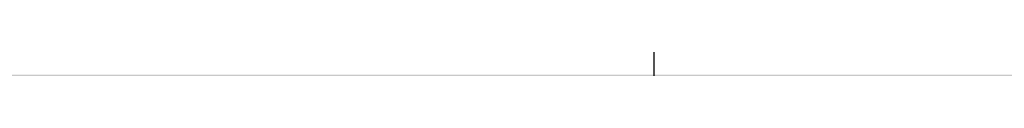
# Model space of a CAD drawing. Units: inches. Extents: x 2083 to 3317, y 1141 to 2115.
# Tile 62 of 256: x 2237.106 to 2238.294, y 1477.769 to 1477.78. Entities that reach past the tile are written whole.
import ezdxf

# ---------------------------------------------------------------- set-up
doc = ezdxf.new("R2010")
doc.units = ezdxf.units.IN
doc.layers.add('A-ANNO-DIMS', color=2, linetype='Continuous', lineweight=18)
doc.layers.add('A-WALL-PATT', color=251, linetype='Continuous', lineweight=13, true_color=0x636466)
doc.styles.get("Standard").update_dxf_attribs({"font": 'arial.ttf'})
doc.dimstyles.new('ISO-25', dxfattribs={"dimtxt": 12, "dimasz": 12, "dimexe": 1.25, "dimexo": 0.625, "dimtad": 1, "dimlunit": 3, "dimtxsty": 'Standard', "dimcen": 2.5, "dimadec": 0, "dimazin": 0, "dimtfac": 1, "dimtmove": 0, "dimatfit": 3, "dimfxl": 1, "dimarcsym": 0})

# ---------------------------------------------------------------- blocks, each defined once
blk = doc.blocks.new('*D30')
at = {"layer": 'A-ANNO-DIMS', "color": 0, "lineweight": -2, "transparency": 16777216}
for p, q in [((2240.0179, 1445.2738), (2240.0179, 1448.0455)), ((2254.3293, 1445.2738), (2254.3293, 1448.0455)), ((2228.0179, 1446.7955), (2216.0179, 1446.7955)), ((2240.0179, 1446.7955), (2254.3293, 1446.7955)), ((2266.3293, 1446.7955), (2413.7649, 1446.7955))]:
    blk.add_line(p, q, dxfattribs=at)
at = {"layer": 'A-ANNO-DIMS', "color": 0, "transparency": 16777216}
for points in [[(2228.0179, 1448.7955), (2228.0179, 1444.7955), (2240.0179, 1446.7955)], [(2266.3293, 1448.7955), (2266.3293, 1444.7955), (2254.3293, 1446.7955)]]:
    blk.add_solid(points, dxfattribs=at)
at = {"layer": 'Defpoints', "color": 0, "transparency": 16777216}
for p in [(2254.3293, 1446.7955), (2240.0179, 1444.6488), (2254.3293, 1444.6488)]:
    blk.add_point(p, dxfattribs=at)
at = {"layer": 'A-ANNO-DIMS', "color": 0, "transparency": 16777216, "insert": (2346.0471, 1453.6252), "char_height": 12, "attachment_point": 5}
blk.add_mtext('WC 1\'-2 1/2" TYP.', dxfattribs=at)
blk = doc.blocks.new('*D31')
at = {"layer": 'A-ANNO-DIMS', "color": 0, "lineweight": -2, "transparency": 16777216}
for p, q in [((2237.8711, 1456.6488), (2237.8711, 1541.9152)), ((2239.3929, 1444.6488), (2236.6211, 1444.6488)), ((2237.8711, 1431.5475), (2237.8711, 1444.6488)), ((2239.3929, 1431.5475), (2236.6211, 1431.5475)), ((2237.8711, 1419.5475), (2237.8711, 1407.5475))]:
    blk.add_line(p, q, dxfattribs=at)
at = {"layer": 'A-ANNO-DIMS', "color": 0, "transparency": 16777216}
for points in [[(2235.8711, 1456.6488), (2239.8711, 1456.6488), (2237.8711, 1444.6488)], [(2235.8711, 1419.5475), (2239.8711, 1419.5475), (2237.8711, 1431.5475)]]:
    blk.add_solid(points, dxfattribs=at)
at = {"layer": 'Defpoints', "color": 0, "transparency": 16777216}
for p in [(2237.8711, 1444.6488), (2240.0179, 1444.6488), (2240.0179, 1431.5475)]:
    blk.add_point(p, dxfattribs=at)
at = {"layer": 'A-ANNO-DIMS', "color": 0, "transparency": 16777216, "insert": (2231.2175, 1505.282), "char_height": 12, "attachment_point": 5, "rotation": 90}
blk.add_mtext('1\'-1" TYP.', dxfattribs=at)
blk = doc.blocks.new('*D45')
at = {"layer": 'A-ANNO-DIMS', "color": 0, "lineweight": -2, "transparency": 16777216}
for p, q in [((2235.9598, 1478.3864), (2235.9598, 1531.3614)), ((2418.9598, 1478.3864), (2418.9598, 1531.3614)), ((2247.9598, 1530.1114), (2406.9598, 1530.1114))]:
    blk.add_line(p, q, dxfattribs=at)
at = {"layer": 'A-ANNO-DIMS', "color": 0, "transparency": 16777216}
for points in [[(2247.9598, 1532.1114), (2247.9598, 1528.1114), (2235.9598, 1530.1114)], [(2406.9598, 1532.1114), (2406.9598, 1528.1114), (2418.9598, 1530.1114)]]:
    blk.add_solid(points, dxfattribs=at)
at = {"layer": 'Defpoints', "color": 0, "transparency": 16777216}
for p in [(2418.9598, 1530.1114), (2235.9598, 1477.7614), (2418.9598, 1477.7614)]:
    blk.add_point(p, dxfattribs=at)
at = {"layer": 'A-ANNO-DIMS', "color": 0, "transparency": 16777216, "insert": (2327.4598, 1536.8673), "char_height": 12, "attachment_point": 5}
blk.add_mtext('15\'-3"', dxfattribs=at)
blk = doc.blocks.new('*D62')
at = {"layer": 'A-ANNO-DIMS', "color": 0, "lineweight": -2, "transparency": 16777216}
for p, q in [((2235.9598, 1469.3864), (2235.9598, 1522.3614)), ((2379.9598, 1469.3864), (2379.9598, 1522.3614)), ((2247.9598, 1521.1114), (2367.9598, 1521.1114))]:
    blk.add_line(p, q, dxfattribs=at)
at = {"layer": 'A-ANNO-DIMS', "color": 0, "transparency": 16777216}
for points in [[(2247.9598, 1523.1114), (2247.9598, 1519.1114), (2235.9598, 1521.1114)], [(2367.9598, 1523.1114), (2367.9598, 1519.1114), (2379.9598, 1521.1114)]]:
    blk.add_solid(points, dxfattribs=at)
at = {"layer": 'Defpoints', "color": 0, "transparency": 16777216}
for p in [(2379.9598, 1521.1114), (2235.9598, 1468.7614), (2379.9598, 1468.7614)]:
    blk.add_point(p, dxfattribs=at)
at = {"layer": 'A-ANNO-DIMS', "color": 0, "transparency": 16777216, "insert": (2307.9598, 1527.8632), "char_height": 12, "attachment_point": 5}
blk.add_mtext('12\'-0"', dxfattribs=at)

msp = doc.modelspace()

# ---------------------------------------------------------------- hatches: boundary and pattern name
at = {"layer": 'A-WALL-PATT'}
h = msp.add_hatch(color=256, dxfattribs=at)
h.dxf.hatch_style = 1
h.paths.add_polyline_path([(3126.9598, 2020.7614), (2748.9598, 2020.7614), (2604.9598, 2020.7614), (2226.9598, 2020.7614), (2226.9598, 1702.7614), (2466.9598, 1702.7614), (2466.9598, 1582.7614), (2418.9598, 1582.7614), (2418.9598, 1477.7614), (2226.9598, 1477.7614), (2226.9598, 1263.2614), (2544.9598, 1263.2614), (2544.9598, 1411.7614), (2604.9598, 1411.7614), (2685.9598, 1411.7614), (2685.9598, 1420.7614), (2604.9598, 1420.7614), (2604.9598, 1573.7614), (2604.9598, 1702.7614), (2604.9598, 2011.7614), (2748.9598, 2011.7614), (2748.9598, 1702.7614), (2862.9598, 1702.7614), (2862.9598, 1621.7614), (2871.9598, 1621.7614), (2871.9598, 1702.7614), (2883.9598, 1702.7614), (2883.9598, 1706.9395, -0.026459), (2883.9598, 1711.7614), (2757.9598, 1711.7614), (2757.9598, 1807.7614), (2787.9598, 1807.7614), (2787.9598, 1812.2614), (2757.9598, 1812.2614), (2757.9598, 2011.7614), (2877.9598, 2011.7614), (2877.9598, 1812.2614), (2847.9598, 1812.2614), (2847.9598, 1807.7614), (2889.8357, 1807.7614), (2889.8357, 1812.2614), (2882.4598, 1812.2614), (2882.4598, 2011.7614), (3117.9598, 2011.7614), (3117.9598, 1812.2614), (2937.8357, 1812.2614), (2937.8357, 1807.7614), (2995.7098, 1807.7614), (2995.7098, 1796.1177), (3000.2098, 1796.1177), (3000.2098, 1807.7614), (3117.9598, 1807.7614), (3117.9598, 1711.7614), (3000.2098, 1711.7614), (3000.2098, 1760.1177), (2998.5727, 1760.1177, -0.020711), (2995.7098, 1760.1177), (2995.7098, 1711.7614), (2931.9598, 1711.7614), (2931.9598, 1702.7614), (3126.9598, 1702.7614)])
h.paths.add_polyline_path([(2471.4598, 2011.7614), (2471.4598, 1810.0114), (2462.7169, 1810.0114), (2462.7169, 1805.5114), (2505.9598, 1805.5114), (2505.9598, 1810.0114), (2475.9598, 1810.0114), (2475.9598, 2011.7614), (2595.9598, 2011.7614), (2595.9598, 1810.0114), (2565.9598, 1810.0114), (2565.9598, 1805.5114), (2595.9598, 1805.5114), (2595.9598, 1711.7614), (2235.9598, 1711.7614), (2235.9598, 1805.5114), (2353.7098, 1805.5114), (2353.7098, 1796.0542), (2358.2098, 1796.0542), (2358.2098, 1805.5114), (2414.7169, 1805.5114), (2414.7169, 1810.0114), (2235.9598, 1810.0114), (2235.9598, 2011.7614)], flags=16)
h.paths.add_polyline_path([(2270.2047, 1994.61), (2270.2047, 1970.61), (2246.2047, 1970.61), (2246.2047, 1994.61)], flags=0)
edge = h.paths.add_edge_path(flags=0)
edge.add_ellipse((2332.0274, 1899.7982), major_axis=(-3.043, 3.043), ratio=0.168252, start_angle=-161.3322, end_angle=-156.3071, ccw=False)
edge.add_ellipse((2333.082, 1898.7435), major_axis=(-1.0546, 1.0546), ratio=0.453532, start_angle=-123.371, end_angle=-94.1591)
edge = h.paths.add_edge_path(flags=0)
edge.add_ellipse((2332.0274, 1968.8763), major_axis=(3.043, 3.043), ratio=0.168252, start_angle=18.6678, end_angle=23.6929)
edge.add_spline(control_points=[(2332.9256, 1970.6911), (2332.2268, 1970.3361), (2330.8937, 1969.6589), (2328.4131, 1970.9321), (2327.2039, 1967.7487), (2324.7096, 1969.9556), (2322.5328, 1967.0124), (2320.0128, 1971.2958), (2317.6803, 1968.1578), (2316.0405, 1967.102), (2315.4269, 1966.8096)], knot_values=[0, 0, 0, 0, 2.267059, 4.324559, 6.685584, 8.878641, 11.121502, 14.300359, 17.755284, 19.732645, 19.732645, 19.732645, 19.732645], degree=3, periodic=0)
edge.add_ellipse((2332.0274, 1968.8763), major_axis=(3.043, 3.043), ratio=0.168252, start_angle=18.6678, end_angle=23.6929, ccw=False)
edge.add_ellipse((2333.082, 1969.9309), major_axis=(1.0546, 1.0546), ratio=0.453532, start_angle=56.629, end_angle=85.8409, ccw=False)
edge = h.paths.add_edge_path(flags=0)
edge.add_spline(control_points=[(2296.4283, 1967.9879), (2293.6278, 1965.3363), (2287.7036, 1959.7271), (2299.7439, 1949.9957), (2294.5326, 1935.6685), (2290.5732, 1920.6035), (2293.3941, 1909.9737), (2296.1854, 1904.9665)], knot_values=[0.099185, 0.099185, 0.099185, 0.099185, 0.345301, 0.619822, 0.982653, 1.386093, 1.810555, 1.810555, 1.810555, 1.810555], degree=3, periodic=0)
edge.add_spline(control_points=[(2296.1854, 1904.9665), (2297.3836, 1902.6193), (2298.001, 1901.9493), (2298.553, 1901.4682)], knot_values=[0.006246, 0.006246, 0.006246, 0.006246, 0.055476, 0.055476, 0.055476, 0.055476], degree=3, periodic=0)
edge.add_spline(control_points=[(2298.553, 1901.4682), (2297.2586, 1900.9232), (2295.2253, 1900.2321), (2293.0602, 1900.6142), (2292.1014, 1900.7884), (2292.0896, 1900.7906)], knot_values=[0.312835, 0.312835, 0.312835, 0.312835, 0.40178, 0.474987, 0.475903, 0.475903, 0.475903, 0.475903], degree=3, periodic=0)
edge.add_arc((2292.7936, 1904.6641), 3.937, 215.4209, 259.6982, ccw=False)
edge.add_spline(control_points=[(2289.5853, 1902.3823), (2289.4767, 1902.5351), (2289.3685, 1902.688), (2289.2609, 1902.8412)], knot_values=[0.102872, 0.102872, 0.102872, 0.102872, 0.116896, 0.116896, 0.116896, 0.116896], degree=3, periodic=0)
edge.add_spline(control_points=[(2289.2609, 1902.8412), (2288.6866, 1902.5502), (2287.64, 1902.0199), (2285.8813, 1901.874), (2283.853, 1901.5044), (2281.72, 1899.7105), (2278.467, 1899.4929), (2276.1571, 1901.8832), (2272.259, 1899.8041), (2267.7776, 1901.8432), (2262.2439, 1900.184), (2257.4149, 1901.7821), (2254.3184, 1900.7261), (2253.1783, 1900.3373)], knot_values=[0, 0, 0, 0, 1.907977, 3.477176, 5.261074, 7.972851, 11.680248, 13.717921, 16.939592, 22.789562, 27.502503, 33.595215, 37.145618, 37.145618, 37.145618, 37.145618], degree=3, periodic=0)
edge.add_line((2253.1783, 1900.3373), (2250.2442, 1902.8412))
edge.add_line((2250.2442, 1902.8412), (2250.2442, 1965.8333))
edge.add_line((2250.2442, 1965.8333), (2253.1783, 1968.3371))
edge.add_spline(control_points=[(2253.1783, 1968.3371), (2254.3184, 1967.9483), (2257.4149, 1966.8924), (2262.2439, 1968.4904), (2267.7776, 1966.8313), (2271.5267, 1968.5372), (2273.8759, 1967.8283), (2274.2067, 1967.7276)], knot_values=[0, 0, 0, 0, 0.09018, 0.244935, 0.364644, 0.513233, 0.537855, 0.537855, 0.537855, 0.537855], degree=3, periodic=0)
edge.add_arc((2274.3529, 1963.7933), 3.937, 72.0511, 92.1279, ccw=False)
edge.add_arc((2281.2969, 1985.23), 18.5963, 252.05113, 288.56572)
edge.add_arc((2292.3167, 1956.0289), 12.6461, 71.02679, 113.77822, ccw=False)
edge = h.paths.add_edge_path(flags=0)
edge.add_spline(control_points=[(2274.8994, 1951.8562), (2275.0662, 1951.6166), (2275.2327, 1951.3766), (2275.398, 1951.1359)], knot_values=[1.409916, 1.409916, 1.409916, 1.409916, 1.43159, 1.43159, 1.43159, 1.43159], degree=3, periodic=0)
edge.add_spline(control_points=[(2275.398, 1951.1359), (2275.7921, 1950.5619), (2276.1792, 1949.9838), (2276.5455, 1949.3971)], knot_values=[1.358238, 1.358238, 1.358238, 1.358238, 1.409916, 1.409916, 1.409916, 1.409916], degree=3, periodic=0)
edge.add_line((2276.5455, 1949.3971), (2277.4373, 1947.8622))
edge.add_spline(control_points=[(2277.4373, 1947.8622), (2276.3038, 1945.6731), (2274.6397, 1942.4269), (2274.6316, 1938.0939), (2272.7991, 1930.8515), (2274.3564, 1943.897), (2275.9477, 1947.9234), (2276.5455, 1949.3971)], knot_values=[0.005632, 0.005632, 0.005632, 0.005632, 0.186014, 0.266002, 0.357087, 0.59639, 0.739732, 0.739732, 0.739732, 0.739732], degree=3, periodic=0)
edge.add_spline(control_points=[(2276.5455, 1949.3971), (2276.1792, 1949.9838), (2275.7921, 1950.5619), (2275.398, 1951.1359)], knot_values=[1.358238, 1.358238, 1.358238, 1.358238, 1.409916, 1.409916, 1.409916, 1.409916], degree=3, periodic=0)
edge.add_spline(control_points=[(2275.398, 1951.1359), (2274.9425, 1950.0805), (2274.2078, 1948.0253), (2273.9346, 1944.8515), (2272.4685, 1937.6275), (2273.4662, 1945.6965), (2274.7006, 1951.0595), (2274.8994, 1951.8562)], knot_values=[0.104364, 0.104364, 0.104364, 0.104364, 0.189636, 0.269624, 0.36071, 0.600013, 0.644622, 0.644622, 0.644622, 0.644622], degree=3, periodic=0)
h.paths.add_polyline_path([(2269.1675, 1963.1276, -0.357527), (2268.1706, 1960.9764, -0.092561), (2268.1706, 1939.4363, -0.357527), (2269.1675, 1937.2851, -0.357527), (2267.0163, 1938.282, -0.164785), (2254.6856, 1938.282, -0.357527), (2252.5344, 1937.2851, -0.357527), (2253.5313, 1939.4363, -0.092561), (2253.5313, 1960.9764, -0.357527), (2252.5344, 1963.1276, -0.357527), (2254.6856, 1962.1307, -0.164785), (2267.0163, 1962.1307, -0.357527)], flags=0)
h.paths.add_polyline_path([(2248.8741, 1967.8018), (2248.8741, 1957.0277), (2249.4578, 1957.0277), (2249.4578, 1911.6468), (2248.8741, 1911.6468), (2248.8741, 1900.8727), (2246.5119, 1900.8727, 0.197327), (2244.1497, 1902.4569), (2244.1497, 1966.2176, 0.197327), (2246.5119, 1967.8018)], flags=0)
h.paths.add_polyline_path([(2269.1675, 1931.3893, -0.357527), (2268.1706, 1929.2381, -0.092561), (2268.1706, 1907.6981, -0.357527), (2269.1675, 1905.5469, -0.357527), (2267.0163, 1906.5438, -0.164785), (2254.6856, 1906.5438, -0.357527), (2252.5344, 1905.5469, -0.357527), (2253.5313, 1907.6981, -0.092561), (2253.5313, 1929.2381, -0.357527), (2252.5344, 1931.3893, -0.357527), (2254.6856, 1930.3925, -0.164785), (2267.0163, 1930.3925, -0.357527)], flags=0)
edge = h.paths.add_edge_path(flags=0)
edge.add_spline(control_points=[(2276.1969, 1906.7237), (2276.1681, 1909.0289), (2276.114, 1913.3719), (2270.5984, 1924.925), (2273.9052, 1919.0128), (2275.9217, 1916.2621), (2275.4746, 1912.4021), (2277.2579, 1910.3806), (2276.696, 1908.225), (2276.6462, 1906.813), (2276.6178, 1906.0084)], knot_values=[0, 0, 0, 0, 8.61026, 16.221274, 18.843057, 23.804898, 27.440828, 29.356102, 31.203478, 33.650687, 33.650687, 33.650687, 33.650687], degree=3, periodic=0)
edge.add_spline(control_points=[(2276.6178, 1906.0084), (2276.6233, 1905.6241), (2276.4977, 1904.6287), (2275.4418, 1903.8547), (2274.9373, 1903.0804), (2274.8591, 1902.8412)], knot_values=[0.156488, 0.156488, 0.156488, 0.156488, 0.184398, 0.231376, 0.250598, 0.250598, 0.250598, 0.250598], degree=3, periodic=0)
edge.add_line((2274.8591, 1902.8412), (2276.506, 1902.8412))
edge.add_spline(control_points=[(2276.506, 1902.8412), (2276.7883, 1903.0849), (2277.6651, 1904.1252), (2278.2495, 1904.3407), (2277.6539, 1908.5274), (2278.1557, 1906.2278), (2278.1005, 1905.2859), (2278.8467, 1904.069), (2277.8568, 1903.4149), (2277.8742, 1902.991), (2277.9036, 1902.8412)], knot_values=[0.059574, 0.059574, 0.059574, 0.059574, 0.080753, 0.103741, 0.16972, 0.176036, 0.207137, 0.240474, 0.262341, 0.27366, 0.27366, 0.27366, 0.27366], degree=3, periodic=0)
edge.add_line((2277.9036, 1902.8412), (2280.0298, 1902.8412))
edge.add_spline(control_points=[(2280.0298, 1902.8412), (2279.8882, 1903.0884), (2279.4993, 1903.9816), (2280.1523, 1905.9393), (2278.1036, 1909.6578), (2279.7624, 1907.1853), (2280.3279, 1904.8749), (2280.4851, 1903.4896), (2281.4633, 1903.2494), (2281.7583, 1902.9365), (2281.834, 1902.8412)], knot_values=[0.013856, 0.013856, 0.013856, 0.013856, 0.034874, 0.088867, 0.107879, 0.126738, 0.158714, 0.193757, 0.217487, 0.226722, 0.226722, 0.226722, 0.226722], degree=3, periodic=0)
edge.add_spline(control_points=[(2281.834, 1902.8412), (2281.7875, 1902.8267), (2281.647, 1902.783), (2281.3955, 1902.8595), (2281.0881, 1902.9852), (2280.7207, 1903.0609), (2280.3335, 1903.0257), (2280.1248, 1902.8989), (2280.0298, 1902.8412)], knot_values=[0, 0, 0, 0, 0.14413, 0.435517, 0.749276, 1.153046, 1.548371, 1.878348, 1.878348, 1.878348, 1.878348], degree=3, periodic=0)
edge.add_line((2280.0298, 1902.8412), (2277.9036, 1902.8412))
edge.add_spline(control_points=[(2277.9036, 1902.8412), (2277.8929, 1902.7959), (2277.8654, 1902.6796), (2277.6075, 1902.6875), (2277.2741, 1902.8007), (2276.8379, 1902.6198), (2276.5838, 1902.7893), (2276.506, 1902.8412)], knot_values=[0, 0, 0, 0, 0.127189, 0.326199, 0.628009, 1.24357, 1.515331, 1.515331, 1.515331, 1.515331], degree=3, periodic=0)
edge.add_line((2276.506, 1902.8412), (2274.8591, 1902.8412))
edge.add_spline(control_points=[(2274.8591, 1902.8412), (2274.8144, 1902.8986), (2274.7251, 1903.0134), (2274.4935, 1903.119), (2274.2443, 1902.9605), (2273.9371, 1903.1849), (2273.614, 1902.9831), (2273.4083, 1902.883), (2273.3223, 1902.8412)], knot_values=[0, 0, 0, 0, 0.21843, 0.436957, 0.687977, 0.990379, 1.398396, 1.69185, 1.69185, 1.69185, 1.69185], degree=3, periodic=0)
edge.add_spline(control_points=[(2273.3223, 1902.8412), (2273.6167, 1903.4457), (2274.274, 1904.5383), (2276.0272, 1904.5737), (2276.207, 1906.5836), (2276.1969, 1906.7237)], knot_values=[0.012227, 0.012227, 0.012227, 0.012227, 0.059472, 0.106218, 0.134458, 0.134458, 0.134458, 0.134458], degree=3, periodic=0)
h.paths.add_polyline_path([(2270.7761, 1897.7898), (2270.7761, 1873.7898), (2246.7761, 1873.7898), (2246.7761, 1897.7898)], flags=0)
h.paths.add_polyline_path([(2353.7098, 1760.0051), (2353.7098, 1760.0542), (2358.2098, 1760.0542, -0.033729)], flags=0)
h.paths.add_polyline_path([(2321.8191, 1737.5292), (2341.9953, 1737.5292, -0.414214), (2343.2033, 1736.3212), (2343.2033, 1721.0206, -0.414214), (2341.9953, 1719.8127), (2321.8191, 1719.8127, -0.414214), (2320.6112, 1721.0206), (2320.6112, 1736.3212, -0.414214)], flags=0)
h.paths.add_polyline_path([(2324.235, 1736.3212), (2339.5794, 1736.3212, -0.414214), (2341.9953, 1733.9053), (2341.9953, 1725.4497, -0.414214), (2339.5794, 1723.0338), (2333.6806, 1723.0338), (2333.8453, 1722.0455, -0.870646), (2335.4254, 1721.8259, -0.767327), (2333.9227, 1721.4232), (2331.291, 1721.4232, -0.767327), (2329.7883, 1721.8259, -0.870646), (2331.3684, 1722.0455), (2331.5331, 1723.0338), (2324.235, 1723.0338, -0.414214), (2321.8191, 1725.4497), (2321.8191, 1733.9053, -0.414214)], flags=0)
h.paths.add_polyline_path([(2570.4838, 1928.6154), (2589.6838, 1928.6154), (2590.1688, 1928.6154), (2590.1688, 1904.9934), (2570.4838, 1904.9934)], flags=0)
h.paths.add_polyline_path([(2574.4473, 1927.2638, -1), (2572.8288, 1927.2638, -1)], flags=0)
h.paths.add_polyline_path([(2573.0899, 1926.9409), (2573.925, 1927.776), (2574.1477, 1927.5533), (2573.3126, 1926.7182)], flags=0)
h.paths.add_polyline_path([(2578.7791, 1919.7296, -1), (2571.5917, 1919.7296, -1)], flags=0)
h.paths.add_polyline_path([(2578.3854, 1919.7296, -1), (2571.9854, 1919.7296, -1)], flags=0)
h.paths.add_polyline_path([(2331.5958, 1729.4762, -1), (2333.618, 1729.4762, -1)], flags=0)
h.paths.add_polyline_path([(2578.0342, 1927.2638, -1), (2576.4157, 1927.2638, -1)], flags=0)
h.paths.add_polyline_path([(2576.6889, 1927.5311), (2576.9116, 1927.7538), (2577.7467, 1926.9186), (2577.524, 1926.6959)], flags=0)
h.paths.add_polyline_path([(2578.1391, 1909.8595, -1), (2572.2317, 1909.8595, -1)], flags=0)
h.paths.add_polyline_path([(2577.7454, 1909.8595, -1), (2572.6254, 1909.8595, -1)], flags=0)
h.paths.add_polyline_path([(2583.7977, 1927.2638, -1), (2582.1792, 1927.2638, -1)], flags=0)
h.paths.add_polyline_path([(2582.7186, 1927.7538), (2583.5538, 1926.9186), (2583.3311, 1926.6959), (2582.4959, 1927.5311)], flags=0)
h.paths.add_polyline_path([(2582.4959, 1927.5311), (2582.7186, 1927.7538), (2583.5538, 1926.9186), (2583.3311, 1926.6959)], flags=0)
h.paths.add_polyline_path([(2587.7391, 1920.5296, -1), (2581.8317, 1920.5296, -1)], flags=0)
h.paths.add_polyline_path([(2587.3454, 1920.5296, -1), (2582.2254, 1920.5296, -1)], flags=0)
h.paths.add_polyline_path([(2587.3846, 1927.2638, -1), (2585.7661, 1927.2638, -1)], flags=0)
h.paths.add_polyline_path([(2586.082, 1926.9802), (2586.9172, 1927.8154), (2587.1399, 1927.5927), (2586.3047, 1926.7575)], flags=0)
h.paths.add_polyline_path([(2588.3791, 1910.6595, -1), (2581.1917, 1910.6595, -1)], flags=0)
h.paths.add_polyline_path([(2587.9854, 1910.6595, -1), (2581.5854, 1910.6595, -1)], flags=0)
h.paths.add_polyline_path([(2417.1677, 1729.4779), (2437.3439, 1729.4779, -0.414214), (2438.5519, 1728.2699), (2438.5519, 1712.9693, -0.414214), (2437.3439, 1711.7614), (2417.1677, 1711.7614, -0.414214), (2415.9598, 1712.9693), (2415.9598, 1728.2699, -0.414214)], flags=0)
h.paths.add_polyline_path([(2419.5836, 1728.2699), (2434.928, 1728.2699, -0.414214), (2437.3439, 1725.8541), (2437.3439, 1717.3984, -0.414214), (2434.928, 1714.9825), (2429.0292, 1714.9825), (2429.1939, 1713.9942, -0.870646), (2430.774, 1713.7746, -0.767327), (2429.2713, 1713.372), (2426.6396, 1713.372, -0.767327), (2425.1369, 1713.7746, -0.870646), (2426.717, 1713.9942), (2426.8817, 1714.9825), (2419.5836, 1714.9825, -0.414214), (2417.1677, 1717.3984), (2417.1677, 1725.8541, -0.414214)], flags=0)
h.paths.add_polyline_path([(2419.5836, 1728.2699), (2434.928, 1728.2699, -0.414214), (2437.3439, 1725.8541), (2437.3439, 1717.3984, -0.414214), (2434.928, 1714.9825), (2429.0292, 1714.9825), (2428.3581, 1719.009), (2427.5528, 1719.009), (2426.8817, 1714.9825), (2419.5836, 1714.9825, -0.414214), (2417.1677, 1717.3984), (2417.1677, 1725.8541, -0.414214)], flags=0)
h.paths.add_polyline_path([(2426.9444, 1721.4249, -1), (2428.9666, 1721.4249, -1)], flags=0)
h.paths.add_polyline_path([(2475.9598, 1702.7614), (2595.9598, 1702.7614), (2595.9598, 1582.7614), (2475.9598, 1582.7614)], flags=16)
h.paths.add_polyline_path([(2427.9598, 1573.7614), (2595.9598, 1573.7614), (2595.9598, 1468.7614), (2595.9598, 1420.7614), (2384.4598, 1420.7614), (2384.4598, 1468.7614), (2427.9598, 1468.7614)], flags=16)
h.paths.add_polyline_path([(2379.9598, 1468.7614), (2379.9598, 1420.7614), (2235.9598, 1420.7614), (2235.9598, 1468.7614)], flags=16)
h.paths.add_polyline_path([(2317.816, 1466.6958), (2337.9922, 1466.6958, -0.414214), (2339.2002, 1465.4878), (2339.2002, 1450.1872, -0.414214), (2337.9922, 1448.9792), (2317.816, 1448.9792, -0.414214), (2316.6081, 1450.1872), (2316.6081, 1465.4878, -0.414214)], flags=0)
h.paths.add_polyline_path([(2320.2319, 1465.4878), (2335.5763, 1465.4878, -0.414214), (2337.9922, 1463.0719), (2337.9922, 1454.6163, -0.414214), (2335.5763, 1452.2004), (2329.6775, 1452.2004), (2329.8422, 1451.212, -0.870646), (2331.4223, 1450.9925, -0.767327), (2329.9196, 1450.5898), (2327.2879, 1450.5898, -0.767327), (2325.7852, 1450.9925, -0.870646), (2327.3653, 1451.212), (2327.53, 1452.2004), (2320.2319, 1452.2004, -0.414214), (2317.816, 1454.6163), (2317.816, 1463.0719, -0.414214)], flags=0)
h.paths.add_polyline_path([(2320.2319, 1465.4878), (2335.5763, 1465.4878, -0.414214), (2337.9922, 1463.0719), (2337.9922, 1454.6163, -0.414214), (2335.5763, 1452.2004), (2329.6775, 1452.2004), (2329.0064, 1456.2269), (2328.2011, 1456.2269), (2327.53, 1452.2004), (2320.2319, 1452.2004, -0.414214), (2317.816, 1454.6163), (2317.816, 1463.0719, -0.414214)], flags=0)
h.paths.add_polyline_path([(2327.5926, 1458.6428, -1), (2329.6148, 1458.6428, -1)], flags=0)
h.paths.add_polyline_path([(2244.4117, 1433.3405), (2241.9209, 1433.3405, -0.414214), (2240.0179, 1435.2435), (2240.0179, 1440.9528, -0.414211), (2241.9209, 1442.8559), (2244.4117, 1442.8559, -1.976472)], flags=0)
h.paths.add_polyline_path([(2245.3569, 1434.3975, -0.414214), (2245.3569, 1441.7988, -2.144098)], flags=0)
h.paths.add_polyline_path([(2535.9598, 1416.2614), (2535.9598, 1272.2614), (2235.9598, 1272.2614), (2235.9598, 1416.2614)], flags=16)
h.paths.add_polyline_path([(2260.1196, 1384.2928), (2260.1196, 1362.0386), (2237.8654, 1362.0386), (2237.8654, 1384.2928)], flags=0)
edge = h.paths.add_edge_path(flags=0)
edge.add_line((2318.2518, 1362.0933), (2318.1458, 1362.001))
edge.add_ellipse((2317.4451, 1360.431), major_axis=(2.8216, 2.8216), ratio=0.168252, start_angle=18.6678, end_angle=20.9481, ccw=False)
edge.add_ellipse((2318.423, 1361.409), major_axis=(0.9779, 0.9779), ratio=0.453532, start_angle=56.629, end_angle=70.2262, ccw=False)
edge = h.paths.add_edge_path(flags=0)
edge.add_line((2319.1074, 1295.5711), (2319.015, 1295.6771))
edge.add_ellipse((2317.4451, 1296.3778), major_axis=(-2.8216, 2.8216), ratio=0.168252, start_angle=-161.3322, end_angle=-159.0519, ccw=False)
edge.add_ellipse((2318.423, 1295.3999), major_axis=(-0.9779, 0.9779), ratio=0.453532, start_angle=-123.371, end_angle=-109.7738)
edge = h.paths.add_edge_path(flags=0)
edge.add_spline(control_points=[(2284.2103, 1301.1702), (2284.5807, 1300.4447), (2284.8912, 1299.892), (2285.1596, 1299.461)], knot_values=[0.039066, 0.039066, 0.039066, 0.039066, 0.055476, 0.055476, 0.055476, 0.055476], degree=3, periodic=0)
edge.add_line((2285.1596, 1299.461), (2284.2103, 1301.1702))
edge = h.paths.add_edge_path(flags=0)
edge.add_line((2280.4125, 1297.298), (2283.37, 1297.0361))
edge.add_line((2283.37, 1297.0361), (2286.4057, 1297.9263))
edge.add_spline(control_points=[(2286.4057, 1297.9263), (2285.3055, 1297.4631), (2284.3448, 1297.1292), (2283.37, 1297.0361)], knot_values=[0.394369, 0.394369, 0.394369, 0.394369, 0.475903, 0.475903, 0.475903, 0.475903], degree=3, periodic=0)
edge.add_spline(control_points=[(2283.37, 1297.0361), (2283.2814, 1297.0277), (2282.3163, 1296.9573), (2281.3125, 1297.1345), (2280.4234, 1297.296), (2280.4125, 1297.298)], knot_values=[0.312835, 0.312835, 0.312835, 0.312835, 0.320246, 0.393453, 0.394369, 0.394369, 0.394369, 0.394369], degree=3, periodic=0)
edge = h.paths.add_edge_path(flags=0)
edge.add_line((2284.4356, 1359.6073), (2280.4463, 1355.328))
edge.add_line((2280.4463, 1355.328), (2279.58, 1351.0178))
edge.add_line((2279.58, 1351.0178), (2282.413, 1346.5804))
edge.add_spline(control_points=[(2282.413, 1346.5804), (2283.1533, 1345.5892), (2284.2529, 1344.0289), (2284.801, 1342.3872), (2284.9352, 1341.8055)], knot_values=[1.240098, 1.240098, 1.240098, 1.240098, 1.332892, 1.382712, 1.382712, 1.382712, 1.382712], degree=3, periodic=0)
edge.add_spline(control_points=[(2284.9352, 1341.8055), (2285.3191, 1340.1406), (2285.233, 1338.4092), (2284.9099, 1336.6541)], knot_values=[1.097484, 1.097484, 1.097484, 1.097484, 1.240098, 1.240098, 1.240098, 1.240098], degree=3, periodic=0)
edge.add_spline(control_points=[(2284.9099, 1336.6541), (2284.5868, 1334.899), (2284.0267, 1333.1203), (2283.4626, 1331.3606)], knot_values=[0.95487, 0.95487, 0.95487, 0.95487, 1.097484, 1.097484, 1.097484, 1.097484], degree=3, periodic=0)
edge.add_line((2283.4626, 1331.3606), (2281.8904, 1326.1534))
edge.add_line((2281.8904, 1326.1534), (2280.7563, 1321.0561))
edge.add_line((2280.7563, 1321.0561), (2280.2992, 1316.002))
edge.add_line((2280.2992, 1316.002), (2280.7159, 1310.9501))
edge.add_line((2280.7159, 1310.9501), (2282.0281, 1305.9721))
edge.add_line((2282.0281, 1305.9721), (2284.2103, 1301.1702))
edge.add_spline(control_points=[(2284.2103, 1301.1702), (2283.3407, 1302.7302), (2282.6119, 1304.3365), (2282.0281, 1305.9721)], knot_values=[0.099185, 0.099185, 0.099185, 0.099185, 0.241799, 0.241799, 0.241799, 0.241799], degree=3, periodic=0)
edge.add_spline(control_points=[(2282.0281, 1305.9721), (2281.4443, 1307.6078), (2281.0055, 1309.2728), (2280.7159, 1310.9501)], knot_values=[0.241799, 0.241799, 0.241799, 0.241799, 0.384413, 0.384413, 0.384413, 0.384413], degree=3, periodic=0)
edge.add_spline(control_points=[(2280.7159, 1310.9501), (2280.4332, 1312.5876), (2280.2894, 1314.277), (2280.2989, 1315.962), (2280.2992, 1316.002)], knot_values=[0.384413, 0.384413, 0.384413, 0.384413, 0.523647, 0.527028, 0.527028, 0.527028, 0.527028], degree=3, periodic=0)
edge.add_spline(control_points=[(2280.2992, 1316.002), (2280.3123, 1317.687), (2280.4779, 1319.3679), (2280.7563, 1321.0561)], knot_values=[0.527028, 0.527028, 0.527028, 0.527028, 0.669642, 0.669642, 0.669642, 0.669642], degree=3, periodic=0)
edge.add_spline(control_points=[(2280.7563, 1321.0561), (2281.0346, 1322.7443), (2281.4259, 1324.4396), (2281.8904, 1326.1534)], knot_values=[0.669642, 0.669642, 0.669642, 0.669642, 0.812256, 0.812256, 0.812256, 0.812256], degree=3, periodic=0)
edge.add_spline(control_points=[(2281.8904, 1326.1534), (2282.2644, 1327.5333), (2282.7879, 1329.2618), (2283.3528, 1331.0178), (2283.4626, 1331.3606)], knot_values=[0.812256, 0.812256, 0.812256, 0.812256, 0.927087, 0.95487, 0.95487, 0.95487, 0.95487], degree=3, periodic=0)
edge.add_line((2283.4626, 1331.3606), (2284.9099, 1336.6541))
edge.add_line((2284.9099, 1336.6541), (2284.9352, 1341.8055))
edge.add_line((2284.9352, 1341.8055), (2282.413, 1346.5804))
edge.add_spline(control_points=[(2282.413, 1346.5804), (2281.2751, 1348.1038), (2280.0784, 1349.5703), (2279.58, 1351.0178)], knot_values=[1.382712, 1.382712, 1.382712, 1.382712, 1.525326, 1.525326, 1.525326, 1.525326], degree=3, periodic=0)
edge.add_spline(control_points=[(2279.58, 1351.0178), (2279.4433, 1351.4147), (2279.1363, 1352.8569), (2279.7352, 1354.2904), (2280.4463, 1355.328)], knot_values=[1.525326, 1.525326, 1.525326, 1.525326, 1.564439, 1.667941, 1.667941, 1.667941, 1.667941], degree=3, periodic=0)
edge.add_spline(control_points=[(2280.4463, 1355.328), (2281.4261, 1356.7578), (2282.9308, 1358.1826), (2284.4356, 1359.6073)], knot_values=[1.667941, 1.667941, 1.667941, 1.667941, 1.810555, 1.810555, 1.810555, 1.810555], degree=3, periodic=0)
edge.add_arc((2280.6231, 1348.5182), 11.7262, 71.02679, 113.77822)
edge.add_arc((2270.4049, 1375.5952), 17.2436, 252.05113, 288.56572, ccw=False)
edge.add_arc((2263.966, 1355.7178), 3.6506, 72.0511, 92.1279)
edge.add_arc((2263.966, 1355.7178), 3.6506, 92.1279, 177.9851)
edge.add_spline(control_points=[(2260.3176, 1355.8462), (2260.2604, 1354.2207), (2260.5513, 1350.1865), (2262.9993, 1346.7663), (2264.4727, 1344.649)], knot_values=[1.43159, 1.43159, 1.43159, 1.43159, 1.564144, 1.770695, 1.770695, 1.770695, 1.770695], degree=3, periodic=0)
edge.add_line((2264.4727, 1344.649), (2264.9356, 1343.9825))
edge.add_spline(control_points=[(2263.801, 1340.2481), (2263.8432, 1340.5141), (2264.0672, 1341.7565), (2264.5127, 1343.0025), (2264.935, 1343.9811)], knot_values=[0.53657, 0.53657, 0.53657, 0.53657, 0.559349, 0.644622, 0.644622, 0.644622, 0.644622], degree=3, periodic=0)
edge.add_spline(control_points=[(2264.935, 1343.9811), (2265.1178, 1343.715), (2265.2989, 1343.4479), (2265.4768, 1343.1794)], knot_values=[1.384077, 1.384077, 1.384077, 1.384077, 1.409916, 1.409916, 1.409916, 1.409916], degree=3, periodic=0)
edge.add_spline(control_points=[(2265.4768, 1343.1794), (2265.6546, 1342.9108), (2265.8293, 1342.6408), (2265.9991, 1342.3688)], knot_values=[1.358238, 1.358238, 1.358238, 1.358238, 1.384077, 1.384077, 1.384077, 1.384077], degree=3, periodic=0)
edge.add_line((2265.9991, 1342.3688), (2266.826, 1340.9455))
edge.add_spline(control_points=[(2266.826, 1340.9455), (2268.8944, 1337.0897), (2271.3982, 1325.843), (2270.5162, 1310.5686), (2275.9194, 1301.8606), (2277.7895, 1299.1994)], knot_values=[0.116896, 0.116896, 0.116896, 0.116896, 0.472987, 1.050969, 1.313793, 1.313793, 1.313793, 1.313793], degree=3, periodic=0)
edge.add_spline(control_points=[(2277.7895, 1299.1994), (2277.8394, 1299.1285), (2277.8894, 1299.0575), (2277.9396, 1298.9866)], knot_values=[0.109884, 0.109884, 0.109884, 0.109884, 0.116896, 0.116896, 0.116896, 0.116896], degree=3, periodic=0)
edge.add_line((2277.9396, 1298.9866), (2277.7888, 1299.1991))
edge.add_spline(control_points=[(2277.7888, 1299.1991), (2277.2566, 1298.9294), (2276.2864, 1298.4379), (2275.0394, 1298.3344), (2274.3833, 1298.2389), (2274.2153, 1298.2093)], knot_values=[33.12187, 33.12187, 33.12187, 33.12187, 35.029056, 36.598255, 37.144827, 37.144827, 37.144827, 37.144827], degree=3, periodic=0)
edge.add_line((2274.2153, 1298.2093), (2273.0731, 1297.893))
edge.add_spline(control_points=[(2273.0731, 1297.893), (2272.3229, 1297.5798), (2271.0392, 1296.5105), (2269.2484, 1296.2261), (2268.4231, 1296.3747)], knot_values=[26.532584, 26.532584, 26.532584, 26.532584, 29.198919, 31.839101, 31.839101, 31.839101, 31.839101], degree=3, periodic=0)
edge.add_line((2268.4231, 1296.3747), (2263.8785, 1297.4575))
edge.add_spline(control_points=[(2263.8785, 1297.4575), (2263.5561, 1297.3594), (2261.8603, 1296.8387), (2260.2388, 1297.2824), (2258.9335, 1297.5165)], knot_values=[15.919551, 15.919551, 15.919551, 15.919551, 16.939592, 21.226067, 21.226067, 21.226067, 21.226067], degree=3, periodic=0)
edge.add_line((2258.9335, 1297.5165), (2254.0552, 1297.329))
edge.add_spline(control_points=[(2254.0552, 1297.329), (2253.7555, 1297.2958), (2252.1137, 1297.1652), (2250.4619, 1297.5442), (2249.1297, 1297.6679)], knot_values=[5.306517, 5.306517, 5.306517, 5.306517, 6.276435, 10.613034, 10.613034, 10.613034, 10.613034], degree=3, periodic=0)
edge.add_line((2249.1297, 1297.6679), (2244.3316, 1296.8778))
edge.add_line((2244.3316, 1296.8778), (2241.611, 1299.1994))
edge.add_line((2241.611, 1299.1994), (2241.611, 1357.6094))
edge.add_line((2241.611, 1357.6094), (2244.3316, 1359.9311))
edge.add_line((2244.3316, 1359.9311), (2252.7288, 1359.5427))
edge.add_spline(control_points=[(2252.7288, 1359.5427), (2252.8709, 1359.5464), (2253.3057, 1359.5482), (2253.7398, 1359.5143), (2254.0317, 1359.4824)], knot_values=[0.233291, 0.233291, 0.233291, 0.233291, 0.244935, 0.268927, 0.268927, 0.268927, 0.268927], degree=3, periodic=0)
edge.add_line((2254.0317, 1359.4824), (2259.5872, 1359.4164))
edge.add_spline(control_points=[(2259.5872, 1359.4164), (2260.6771, 1359.6285), (2262.0732, 1359.897), (2263.5237, 1359.4593), (2263.8304, 1359.366)], knot_values=[0.422516, 0.422516, 0.422516, 0.422516, 0.513233, 0.537855, 0.537855, 0.537855, 0.537855], degree=3, periodic=0)
edge.add_arc((2263.966, 1355.7178), 3.6506, 72.0511, 92.1279, ccw=False)
edge.add_arc((2270.4049, 1375.5952), 17.2436, 252.05113, 288.56572)
edge.add_arc((2280.6231, 1348.5182), 11.7262, 71.02679, 113.77822, ccw=False)
h.paths.add_polyline_path([(2240.3405, 1359.4347), (2240.3405, 1349.4444), (2240.8818, 1349.4444), (2240.8818, 1307.3645), (2240.3405, 1307.3645), (2240.3405, 1297.3741), (2238.1502, 1297.3741, 0.197327), (2235.9598, 1298.8431), (2235.9598, 1357.9657, 0.197327), (2238.1502, 1359.4347)], flags=0)
h.paths.add_polyline_path([(2259.1578, 1355.1005, -0.357527), (2258.2334, 1353.1058, -0.092561), (2258.2334, 1333.1326, -0.357527), (2259.1578, 1331.1379, -0.357527), (2257.1631, 1332.0622, -0.164785), (2245.7293, 1332.0622, -0.357527), (2243.7346, 1331.1379, -0.357527), (2244.6589, 1333.1326, -0.092561), (2244.6589, 1353.1058, -0.357527), (2243.7346, 1355.1005, -0.357527), (2245.7293, 1354.1761, -0.164785), (2257.1631, 1354.1761, -0.357527)], flags=0)
edge = h.paths.add_edge_path(flags=0)
edge.add_line((2265.9991, 1342.3688), (2266.826, 1340.9455))
edge.add_line((2266.826, 1340.9455), (2265.3076, 1337.8141))
edge.add_line((2265.3076, 1337.8141), (2264.3582, 1334.6529))
edge.add_line((2264.3582, 1334.6529), (2264.262, 1333.7997))
edge.add_spline(control_points=[(2264.262, 1333.7997), (2264.2084, 1333.1871), (2264.1621, 1332.3655), (2264.0071, 1331.4139), (2263.969, 1331.2018)], knot_values=[0.464444, 0.464444, 0.464444, 0.464444, 0.516691, 0.531608, 0.531608, 0.531608, 0.531608], degree=3, periodic=0)
edge.add_spline(control_points=[(2263.969, 1331.2018), (2263.7745, 1330.1189), (2263.4244, 1328.7908), (2263.2574, 1328.5307), (2263.234, 1328.5146)], knot_values=[0.372682, 0.372682, 0.372682, 0.372682, 0.44885, 0.464444, 0.464444, 0.464444, 0.464444], degree=3, periodic=0)
edge.add_spline(control_points=[(2263.234, 1328.5146), (2263.0964, 1328.4202), (2263.1312, 1329.3015), (2263.275, 1330.6157)], knot_values=[0.280919, 0.280919, 0.280919, 0.280919, 0.372682, 0.372682, 0.372682, 0.372682], degree=3, periodic=0)
edge.add_spline(control_points=[(2263.275, 1330.6157), (2263.4187, 1331.93), (2263.6715, 1333.6773), (2263.9699, 1335.315)], knot_values=[0.189157, 0.189157, 0.189157, 0.189157, 0.280919, 0.280919, 0.280919, 0.280919], degree=3, periodic=0)
edge.add_spline(control_points=[(2263.9699, 1335.315), (2264.1005, 1336.0322), (2264.4188, 1337.6219), (2264.7548, 1338.8644), (2264.9474, 1339.4911)], knot_values=[0.097394, 0.097394, 0.097394, 0.097394, 0.137578, 0.189157, 0.189157, 0.189157, 0.189157], degree=3, periodic=0)
edge.add_spline(control_points=[(2264.9474, 1339.4911), (2265.29, 1340.6061), (2265.6442, 1341.494), (2265.9991, 1342.3688)], knot_values=[0.005632, 0.005632, 0.005632, 0.005632, 0.097394, 0.097394, 0.097394, 0.097394], degree=3, periodic=0)
h.paths.add_polyline_path([(2259.1578, 1325.671, -0.357527), (2258.2334, 1323.6763, -0.092561), (2258.2334, 1303.7031, -0.357527), (2259.1578, 1301.7084, -0.357527), (2257.1631, 1302.6327, -0.164785), (2245.7293, 1302.6327, -0.357527), (2243.7346, 1301.7084, -0.357527), (2244.6589, 1303.7031, -0.092561), (2244.6589, 1323.6763, -0.357527), (2243.7346, 1325.671, -0.357527), (2245.7293, 1324.7466, -0.164785), (2257.1631, 1324.7466, -0.357527)], flags=0)
edge = h.paths.add_edge_path(flags=0)
edge.add_spline(control_points=[(2261.7089, 1317.3114), (2261.6795, 1317.4176), (2261.7619, 1317.3885), (2262.4907, 1316.0899), (2262.9622, 1315.3009)], knot_values=[14.955861, 14.955861, 14.955861, 14.955861, 16.221274, 18.694826, 18.694826, 18.694826, 18.694826], degree=3, periodic=0)
edge.add_spline(control_points=[(2262.9622, 1315.3009), (2262.9904, 1315.2536), (2263.7021, 1314.0674), (2264.349, 1313.1272), (2264.7301, 1312.1642)], knot_values=[18.694826, 18.694826, 18.694826, 18.694826, 18.843057, 22.433791, 22.433791, 22.433791, 22.433791], degree=3, periodic=0)
edge.add_spline(control_points=[(2264.7301, 1312.1642), (2264.8756, 1311.7964), (2265.1769, 1310.7698), (2265.1431, 1309.5593), (2265.2477, 1308.8242)], knot_values=[22.433791, 22.433791, 22.433791, 22.433791, 23.804898, 26.172756, 26.172756, 26.172756, 26.172756], degree=3, periodic=0)
edge.add_line((2265.2477, 1308.8242), (2265.8508, 1307.1719))
edge.add_spline(control_points=[(2265.8508, 1307.1719), (2266.065, 1306.8217), (2266.3844, 1306.3322), (2266.4244, 1305.7805), (2266.4204, 1305.6112)], knot_values=[28.062562, 28.062562, 28.062562, 28.062562, 29.356102, 29.911721, 29.911721, 29.911721, 29.911721], degree=3, periodic=0)
edge.add_spline(control_points=[(2266.4204, 1305.6112), (2266.4161, 1305.4326), (2266.394, 1305.25), (2266.3648, 1305.0659)], knot_values=[29.911721, 29.911721, 29.911721, 29.911721, 30.497837, 30.497837, 30.497837, 30.497837], degree=3, periodic=0)
edge.add_line((2266.3648, 1305.0659), (2266.0662, 1302.1363))
edge.add_spline(control_points=[(2266.0662, 1302.1363), (2266.0712, 1301.78), (2265.9981, 1301.2), (2265.6633, 1300.759), (2265.5089, 1300.5859)], knot_values=[0.156488, 0.156488, 0.156488, 0.156488, 0.184398, 0.203543, 0.203543, 0.203543, 0.203543], degree=3, periodic=0)
edge.add_line((2265.5089, 1300.5859), (2264.4353, 1299.1994))
edge.add_line((2264.4353, 1299.1994), (2265.9624, 1299.1994))
edge.add_line((2265.9624, 1299.1994), (2267.336, 1301.1753))
edge.add_line((2267.336, 1301.1753), (2267.3117, 1301.9862))
edge.add_spline(control_points=[(2267.3117, 1301.9862), (2267.2611, 1302.8624), (2267.1602, 1303.7371), (2267.2715, 1303.3259)], knot_values=[0.126229, 0.126229, 0.126229, 0.126229, 0.166617, 0.166617, 0.166617, 0.166617], degree=3, periodic=0)
edge.add_spline(control_points=[(2267.2715, 1303.3259), (2267.28, 1303.2943), (2267.3098, 1303.1754), (2267.3735, 1302.8836), (2267.4061, 1302.6828), (2267.4179, 1302.601)], knot_values=[0.166617, 0.166617, 0.166617, 0.166617, 0.16972, 0.176036, 0.180765, 0.180765, 0.180765, 0.180765], degree=3, periodic=0)
edge.add_spline(control_points=[(2267.7439, 1300.9875), (2267.6876, 1301.1509), (2267.4805, 1301.6567), (2267.4838, 1302.1448), (2267.4179, 1302.601)], knot_values=[0.180765, 0.180765, 0.180765, 0.180765, 0.193767, 0.220139, 0.220139, 0.220139, 0.220139], degree=3, periodic=0)
edge.add_line((2267.4179, 1302.601), (2267.7439, 1300.9875))
edge.add_spline(control_points=[(2267.7439, 1300.9875), (2267.832, 1300.7319), (2267.932, 1300.3099), (2267.5548, 1299.9745), (2267.4294, 1299.8292)], knot_values=[0.220139, 0.220139, 0.220139, 0.220139, 0.240474, 0.25489, 0.25489, 0.25489, 0.25489], degree=3, periodic=0)
edge.add_line((2267.4294, 1299.8292), (2267.2584, 1299.1994))
edge.add_line((2267.2584, 1299.1994), (2269.23, 1299.1994))
edge.add_spline(control_points=[(2269.23, 1299.1994), (2269.0987, 1299.4287), (2268.8428, 1300.0163), (2269.0116, 1300.9159), (2268.9468, 1301.6607)], knot_values=[0.013856, 0.013856, 0.013856, 0.013856, 0.034874, 0.067073, 0.067073, 0.067073, 0.067073], degree=3, periodic=0)
edge.add_line((2268.9468, 1301.6607), (2268.4316, 1303.6031))
edge.add_spline(control_points=[(2268.4316, 1303.6031), (2268.1756, 1304.1924), (2267.5962, 1305.2513), (2268.0407, 1304.6232), (2268.2514, 1304.2824)], knot_values=[0.090155, 0.090155, 0.090155, 0.090155, 0.107879, 0.120289, 0.120289, 0.120289, 0.120289], degree=3, periodic=0)
edge.add_spline(control_points=[(2268.2514, 1304.2824), (2268.3609, 1304.1053), (2269.0578, 1302.918), (2269.3827, 1301.5904), (2269.5214, 1300.7759), (2269.5752, 1300.5558)], knot_values=[0.120289, 0.120289, 0.120289, 0.120289, 0.126738, 0.158714, 0.173506, 0.173506, 0.173506, 0.173506], degree=3, periodic=0)
edge.add_line((2269.5752, 1300.5558), (2270.6858, 1299.4213))
edge.add_spline(control_points=[(2270.6858, 1299.4213), (2270.7672, 1299.3573), (2270.8379, 1299.2814), (2270.9029, 1299.1994)], knot_values=[0.21816, 0.21816, 0.21816, 0.21816, 0.226722, 0.226722, 0.226722, 0.226722], degree=3, periodic=0)
edge.add_line((2270.9372, 1299.1929), (2270.9029, 1299.1994))
edge.add_spline(control_points=[(2270.9029, 1299.1994), (2270.8598, 1299.186), (2270.7295, 1299.1455), (2270.4963, 1299.2164), (2270.2717, 1299.3083), (2270.121, 1299.348), (2270.0633, 1299.3596)], knot_values=[0.939174, 0.939174, 0.939174, 0.939174, 1.083304, 1.374691, 1.68845, 1.878348, 1.878348, 1.878348, 1.878348], degree=3, periodic=0)
edge.add_line((2270.0633, 1299.3596), (2269.23, 1299.1994))
edge.add_line((2269.23, 1299.1994), (2267.2584, 1299.1994))
edge.add_spline(control_points=[(2267.2584, 1299.1994), (2267.2484, 1299.1574), (2267.223, 1299.0497), (2266.9838, 1299.0569), (2266.8092, 1299.1162), (2266.6769, 1299.1091), (2266.6365, 1299.1048)], knot_values=[0.757665, 0.757665, 0.757665, 0.757665, 0.884854, 1.083864, 1.385675, 1.515331, 1.515331, 1.515331, 1.515331], degree=3, periodic=0)
edge.add_spline(control_points=[(2266.6365, 1299.1048), (2266.4852, 1299.0888), (2266.2358, 1299.0171), (2266.0346, 1299.1513), (2265.9624, 1299.1994)], knot_values=[0, 0, 0, 0, 0.485905, 0.757665, 0.757665, 0.757665, 0.757665], degree=3, periodic=0)
edge.add_line((2265.9624, 1299.1994), (2264.4353, 1299.1994))
edge.add_line((2264.4353, 1299.1994), (2263.8584, 1299.3671))
edge.add_spline(control_points=[(2263.8584, 1299.3671), (2263.8189, 1299.3709), (2263.7795, 1299.3857), (2263.7401, 1299.4015)], knot_values=[0.845925, 0.845925, 0.845925, 0.845925, 0.978627, 0.978627, 0.978627, 0.978627], degree=3, periodic=0)
edge.add_line((2263.7218, 1299.3964), (2263.0103, 1299.1994))
edge.add_spline(control_points=[(2263.0103, 1299.1994), (2263.2458, 1299.6829), (2263.506, 1300.1281), (2263.8735, 1300.408)], knot_values=[0.012227, 0.012227, 0.012227, 0.012227, 0.052971, 0.052971, 0.052971, 0.052971], degree=3, periodic=0)
edge.add_spline(control_points=[(2263.8735, 1300.408), (2263.9321, 1300.4527), (2264.0842, 1300.553), (2264.2552, 1300.6242), (2264.3597, 1300.6647)], knot_values=[0.052971, 0.052971, 0.052971, 0.052971, 0.059472, 0.069086, 0.069086, 0.069086, 0.069086], degree=3, periodic=0)
edge.add_line((2264.3597, 1300.6647), (2265.1419, 1301.0778))
edge.add_line((2265.1419, 1301.0778), (2265.6758, 1302.7996))
edge.add_line((2265.6758, 1302.7996), (2265.5407, 1305.7041))
edge.add_line((2265.5407, 1305.7041), (2264.8031, 1309.3277))
edge.add_line((2264.8031, 1309.3277), (2263.0405, 1314.0918))
edge.add_spline(control_points=[(2263.0405, 1314.0918), (2262.3836, 1315.6714), (2261.796, 1316.9977), (2261.7089, 1317.3114)], knot_values=[11.216896, 11.216896, 11.216896, 11.216896, 14.955861, 14.955861, 14.955861, 14.955861], degree=3, periodic=0)
h.paths.add_polyline_path([(2871.9598, 1416.2614), (2895.91, 1416.2614), (2895.91, 1420.7614), (2871.9598, 1420.7614), (2871.9598, 1501.7614), (2862.9598, 1501.7614), (2862.9598, 1420.7614), (2805.9598, 1420.7614), (2805.9598, 1411.7614), (2862.9598, 1411.7614), (2862.9598, 1263.2614), (3126.9598, 1263.2614), (3126.9598, 1411.7614), (3126.9598, 1486.7614), (2943.9598, 1486.7614), (2943.9598, 1477.7614), (2967.8603, 1477.7614), (2967.8603, 1420.7614), (2943.91, 1420.7614), (2943.91, 1416.2614), (3117.9598, 1416.2614), (3117.9598, 1420.7614), (2972.3603, 1420.7614), (2972.3603, 1477.7614), (3117.9598, 1477.7614), (3117.9598, 1420.7614), (3117.9598, 1272.2614), (2871.9598, 1272.2614)], flags=0)
h.paths.add_polyline_path([(2457.1256, 1485.9425), (2527.6027, 1485.9425), (2527.6027, 1537.6357), (2457.1256, 1537.6357)], flags=8)
h.paths.add_polyline_path([(2481.0051, 1609.9818), (2590.7658, 1609.9818), (2590.7658, 1682.0034), (2481.0051, 1682.0034)], flags=8)
h.paths.add_polyline_path([(2483.085, 1729.1268), (2553.562, 1729.1268), (2553.562, 1780.82), (2483.085, 1780.82)], flags=8)

# ---------------------------------------------------------------- dimensions: what is measured, and where the dimension line sits
at = {"layer": 'A-ANNO-DIMS'}
for base, p1, p2, picture, middle in [((2418.9598, 1530.1114), (2235.9598, 1477.7614), (2418.9598, 1477.7614), '*D45', (2327.4598, 1536.8673)), ((2379.9598, 1521.1114), (2235.9598, 1468.7614), (2379.9598, 1468.7614), '*D62', (2307.9598, 1527.8632))]:
    dim = msp.add_linear_dim(base=base, p1=p1, p2=p2, dimstyle='ISO-25', override={"dimdec": 1, "dimlfac": 1, "dimrnd": 0, "dimzin": 1, "dimdsep": 46, "dimlunit": 4, "dimfrac": 2}, dxfattribs=at)
    dim.commit()
    dim.dimension.update_dxf_attribs({"geometry": picture, "text_midpoint": middle})
dim = msp.add_linear_dim(base=(2237.8711, 1444.6488), p1=(2240.0179, 1431.5475), p2=(2240.0179, 1444.6488), angle=90, text='<> TYP.', dimstyle='ISO-25', override={"dimdec": 1, "dimlfac": 1, "dimrnd": 0, "dimzin": 1, "dimdsep": 46, "dimlunit": 4, "dimfrac": 2}, dxfattribs=at)
dim.commit()
dim.dimension.update_dxf_attribs({"geometry": '*D31', "text_midpoint": (2231.2175, 1505.282)})
dim = msp.add_linear_dim(base=(2254.3293, 1446.7955), p1=(2240.0179, 1444.6488), p2=(2254.3293, 1444.6488), text='WC <> TYP.', dimstyle='ISO-25', override={"dimdec": 1, "dimlfac": 1, "dimrnd": 0, "dimzin": 1, "dimdsep": 46, "dimlunit": 4, "dimfrac": 2}, dxfattribs=at)
dim.commit()
dim.dimension.update_dxf_attribs({"geometry": '*D30', "text_midpoint": (2346.0471, 1453.6252)})

doc.saveas('drawing.dxf')
